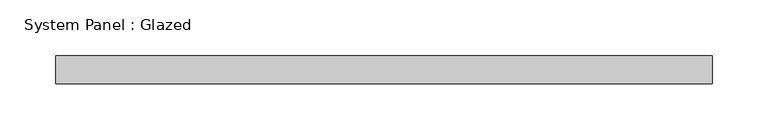
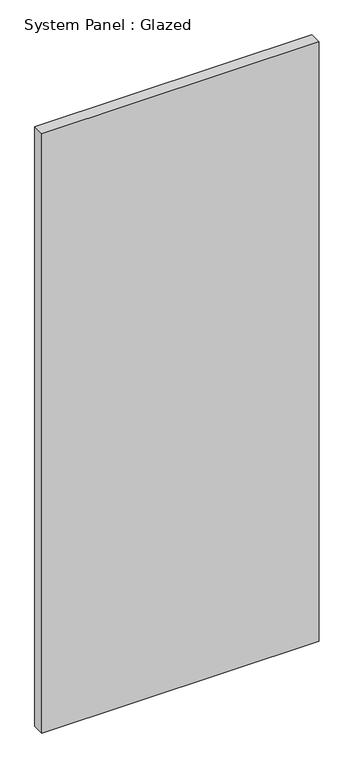
"""IFC4 building model written with IfcOpenShell, lengths in millimetres: plate geometry, System Panel : Glazed."""

from ifc_helpers import new_model, si_unit, origin, origin_with_axes, place, context, project, spatial, polyline, outline, extrude, source, transform, mapped, element, save


def system_panel_glazed_a8526af5(model_context):
    return source(origin(), model_context, "Body", "SweptSolid", [
        extrude(outline(polyline([(295.275, 19.05), (-295.275, 19.05), (-295.275, 44.45), (295.275, 44.45), (295.275, 19.05)])), origin_with_axes(), (0.0, 0.0, 1.0), 1348.7821201),
    ])


if __name__ == "__main__":
    model = new_model("IFC4")
    model_context = context("Model", 3, world=origin())
    ifc_project = project(units=[si_unit("LENGTHUNIT", "METRE", prefix="MILLI")], contexts=[model_context])
    site = spatial("IfcSite", under=ifc_project)
    building = spatial("IfcBuilding", under=site)
    placement = place(None, origin())
    system_panel_glazed_shape = system_panel_glazed_a8526af5(model_context)
    element("IfcPlate", 1, ObjectType="System Panel : Glazed", at=placement, inside=building, context=model_context, shape_type="MappedRepresentation", body=[
        mapped(system_panel_glazed_shape, transform((0.0, 0.0, 0.0), x_axis=(1.0, 0.0, 0.0), y_axis=(0.0, 1.0, 0.0), z_axis=(0.0, 0.0, 1.0))),
    ])
    save(model, "model.ifc")

# Revit data of these elements
# Type "System Panel : Glazed"
#   Construction Type Id = "GSP4R"
#   Analytic Construction = "1/8 in Pilkington single glazing"
#   Visual Light Transmittance = 0.9
#   Solar Heat Gain Coefficient = 0.86
#   Heat Transfer Coefficient (U) = 1.18115 BTU/(h·ft²·°F)
#   Define Thermal Properties by = 1
# Element 1 (IfcPlate, "System Panel : Glazed")
#   Materials on its faces: "Glass"
# Materials
#   "Glass": class "Glass", colour RGB 0 128 192, transparency 0.75, Description = "Soda Lime Glass", Cost = 0
